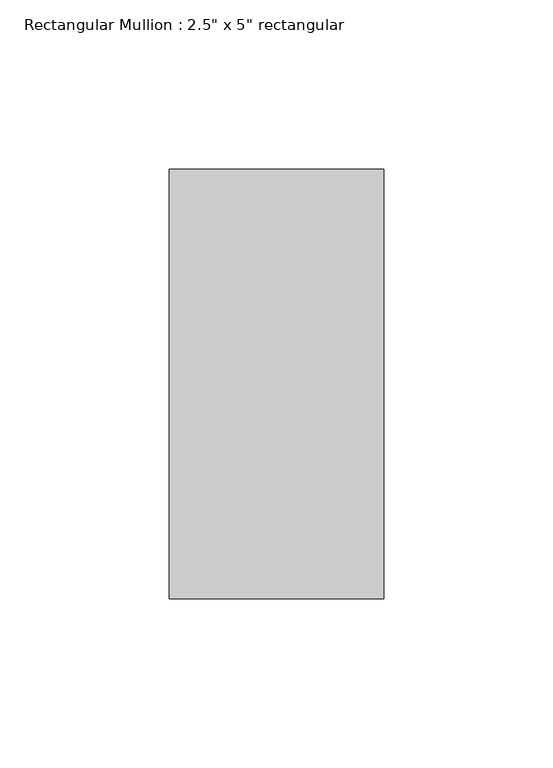
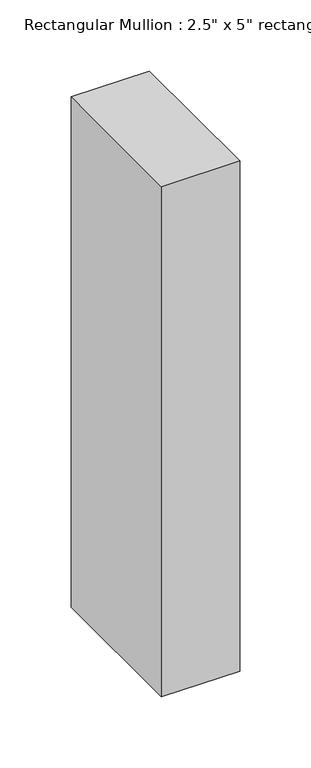
"""IFC4 building model written with IfcOpenShell, lengths in millimetres: member geometry."""

from ifc_helpers import new_model, si_unit, frame, origin, place, context, project, spatial, polyline, outline, extrude, source, transform, mapped, element, save


def member_505fbe18(model_context):
    return source(origin(), model_context, "Body", "SweptSolid", [
        extrude(outline(polyline([(31.75, 63.5), (31.75, -63.5), (-31.75, -63.5), (-31.75, 63.5), (31.75, 63.5)])), frame((0.0, 0.0, -438.15), z_axis=(0.0, 0.0, 1.0), x_axis=(1.0, 0.0, 0.0)), (0.0, 0.0, 1.0), 438.15),
    ])


if __name__ == "__main__":
    model = new_model("IFC4")
    model_context = context("Model", 3, world=origin())
    ifc_project = project(units=[si_unit("LENGTHUNIT", "METRE", prefix="MILLI")], contexts=[model_context])
    site = spatial("IfcSite", under=ifc_project)
    building = spatial("IfcBuilding", under=site)
    placement = place(None, origin())
    member_shape = member_505fbe18(model_context)
    element("IfcMember", 1, ObjectType="Rectangular Mullion : 2.5\" x 5\" rectangular", at=placement, inside=building, context=model_context, shape_type="MappedRepresentation", body=[
        mapped(member_shape, transform((0.0, 0.0, 0.0), x_axis=(1.0, 0.0, 0.0), y_axis=(0.0, 1.0, 0.0), z_axis=(0.0, 0.0, 1.0))),
    ])
    save(model, "model.ifc")

# Revit data of these elements
# Type "Rectangular Mullion : 2.5\" x 5\" rectangular"
#   built-in parameter 1007304 = 0.416667 (stored number, unit not read)
#   built-in parameter 1007301 = 0.104167 (stored number, unit not read)
#   built-in parameter 1007300 = 0.104167 (stored number, unit not read)
# Element 1 (IfcMember, "Rectangular Mullion : 2.5\" x 5\" rectangular")
#   Materials on its faces: "Aluminum"
# Materials
#   "Aluminum": class "Metal", colour RGB 247 247 247, transparency 0, Description = "Aluminum 6061", Cost = 0
